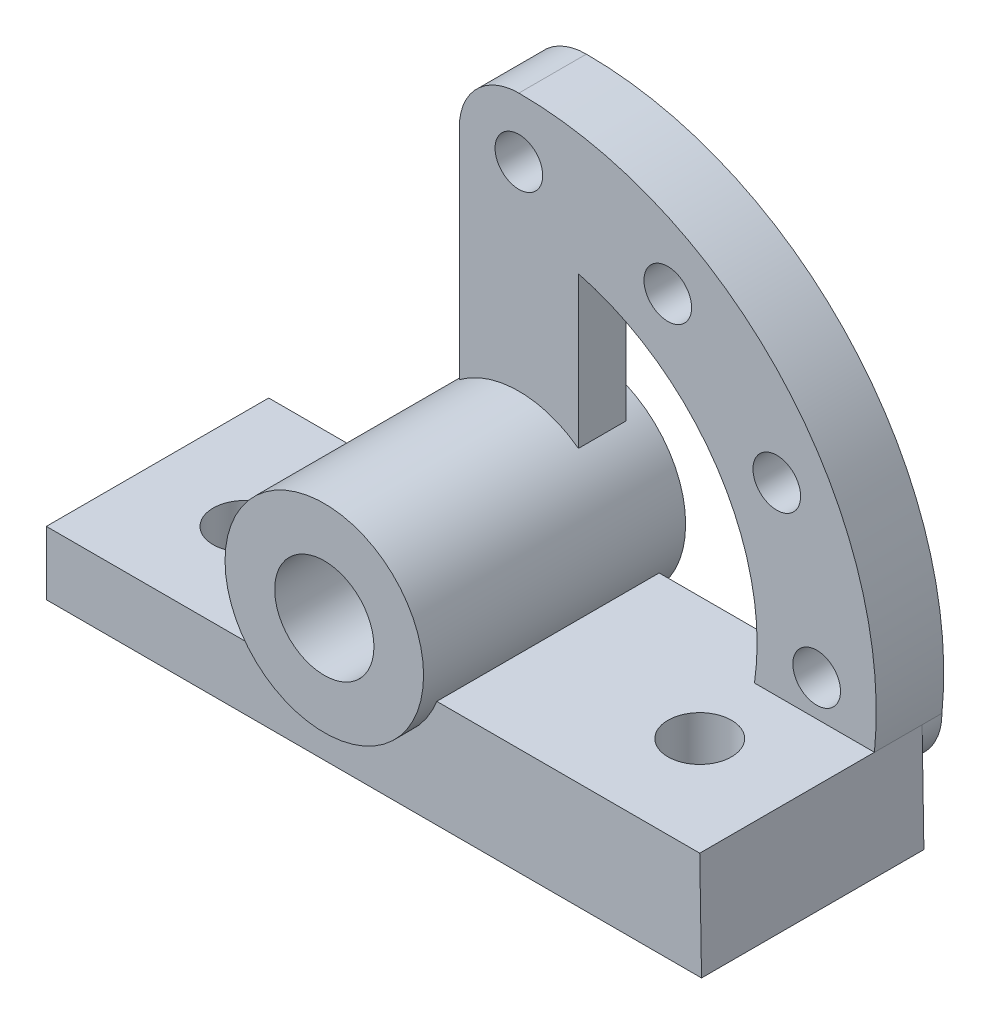
ISO-10303-21;
HEADER;
FILE_DESCRIPTION(('STEP AP214'),'2;1');
FILE_NAME('part.step','',(''),(''),'','','');
FILE_SCHEMA(('AUTOMOTIVE_DESIGN { 1 0 10303 214 1 1 1 1 }'));
ENDSEC;
DATA;
#1=APPLICATION_CONTEXT('core data for automotive mechanical design processes');
#2=APPLICATION_PROTOCOL_DEFINITION('international standard','automotive_design',2000,#1);
#3=PRODUCT_CONTEXT('',#1,'mechanical');
#4=PRODUCT('Part','Part','',(#3));
#5=PRODUCT_RELATED_PRODUCT_CATEGORY('part','',(#4));
#6=PRODUCT_DEFINITION_FORMATION('','',#4);
#7=PRODUCT_DEFINITION_CONTEXT('part definition',#1,'design');
#8=PRODUCT_DEFINITION('design','',#6,#7);
#9=PRODUCT_DEFINITION_SHAPE('','',#8);
#10=(LENGTH_UNIT() NAMED_UNIT(*) SI_UNIT(.MILLI.,.METRE.));
#11=(NAMED_UNIT(*) PLANE_ANGLE_UNIT() SI_UNIT($,.RADIAN.));
#12=(NAMED_UNIT(*) SI_UNIT($,.STERADIAN.) SOLID_ANGLE_UNIT());
#13=UNCERTAINTY_MEASURE_WITH_UNIT(LENGTH_MEASURE(1.E-05),#10,'distance_accuracy_value','');
#14=(GEOMETRIC_REPRESENTATION_CONTEXT(3) GLOBAL_UNCERTAINTY_ASSIGNED_CONTEXT((#13)) GLOBAL_UNIT_ASSIGNED_CONTEXT((#10,
#11,#12)) REPRESENTATION_CONTEXT('',''));
#15=CARTESIAN_POINT('',(0.,0.,0.));
#16=DIRECTION('',(0.,0.,1.));
#17=DIRECTION('',(1.,0.,0.));
#18=AXIS2_PLACEMENT_3D('',#15,#16,#17);
#19=CARTESIAN_POINT('',(75.,36.,-5.));
#20=DIRECTION('',(0.,0.,1.));
#21=DIRECTION('',(1.,0.,0.));
#22=AXIS2_PLACEMENT_3D('',#19,#20,#21);
#23=CYLINDRICAL_SURFACE('',#22,12.5);
#24=CARTESIAN_POINT('',(75.,36.,-5.));
#25=DIRECTION('',(0.,0.,1.));
#26=DIRECTION('',(1.,0.,0.));
#27=AXIS2_PLACEMENT_3D('',#24,#25,#26);
#28=CIRCLE('',#27,12.5);
#29=CARTESIAN_POINT('',(87.5,36.,-5.));
#30=VERTEX_POINT('',#29);
#31=EDGE_CURVE('E313',#30,#30,#28,.T.);
#32=ORIENTED_EDGE('',*,*,#31,.F.);
#33=EDGE_LOOP('',(#32));
#34=FACE_BOUND('',#33,.T.);
#35=CARTESIAN_POINT('',(75.,36.,61.));
#36=DIRECTION('',(0.,0.,1.));
#37=DIRECTION('',(1.,0.,0.));
#38=AXIS2_PLACEMENT_3D('',#35,#36,#37);
#39=CIRCLE('',#38,12.5);
#40=CARTESIAN_POINT('',(87.5,36.,61.));
#41=VERTEX_POINT('',#40);
#42=EDGE_CURVE('E308',#41,#41,#39,.T.);
#43=ORIENTED_EDGE('',*,*,#42,.T.);
#44=EDGE_LOOP('',(#43));
#45=FACE_BOUND('',#44,.T.);
#46=ADVANCED_FACE('F41',(#34,#45),#23,.F.);
#47=CARTESIAN_POINT('',(75.,36.,-5.));
#48=DIRECTION('',(0.,0.,1.));
#49=DIRECTION('',(1.,0.,0.));
#50=AXIS2_PLACEMENT_3D('',#47,#48,#49);
#51=CYLINDRICAL_SURFACE('',#50,25.);
#52=CARTESIAN_POINT('',(75.,36.,12.));
#53=DIRECTION('',(0.,0.,1.));
#54=DIRECTION('',(1.,0.,0.));
#55=AXIS2_PLACEMENT_3D('',#52,#53,#54);
#56=CIRCLE('',#55,25.);
#57=CARTESIAN_POINT('',(90.,56.,12.));
#58=VERTEX_POINT('',#57);
#59=CARTESIAN_POINT('',(60.,56.,12.));
#60=VERTEX_POINT('',#59);
#61=EDGE_CURVE('E171',#58,#60,#56,.T.);
#62=ORIENTED_EDGE('',*,*,#61,.T.);
#63=DIRECTION('',(0.,0.,-1.));
#64=VECTOR('',#63,1.);
#65=CARTESIAN_POINT('',(60.,56.,12.));
#66=LINE('',#65,#64);
#67=CARTESIAN_POINT('',(60.,56.,0.));
#68=VERTEX_POINT('',#67);
#69=EDGE_CURVE('E155',#60,#68,#66,.T.);
#70=ORIENTED_EDGE('',*,*,#69,.T.);
#71=CARTESIAN_POINT('',(75.,36.,0.));
#72=DIRECTION('',(0.,0.,1.));
#73=DIRECTION('',(1.,0.,0.));
#74=AXIS2_PLACEMENT_3D('',#71,#72,#73);
#75=CIRCLE('',#74,25.);
#76=CARTESIAN_POINT('',(90.,56.,0.));
#77=VERTEX_POINT('',#76);
#78=EDGE_CURVE('E192',#77,#68,#75,.T.);
#79=ORIENTED_EDGE('',*,*,#78,.F.);
#80=DIRECTION('',(0.,0.,-1.));
#81=VECTOR('',#80,1.);
#82=CARTESIAN_POINT('',(90.,56.,12.));
#83=LINE('',#82,#81);
#84=EDGE_CURVE('E165',#58,#77,#83,.T.);
#85=ORIENTED_EDGE('',*,*,#84,.F.);
#86=EDGE_LOOP('',(#62,#70,#79,#85));
#87=FACE_BOUND('',#86,.T.);
#88=CARTESIAN_POINT('',(75.,36.,56.));
#89=DIRECTION('',(0.,0.,1.));
#90=DIRECTION('',(1.,0.,0.));
#91=AXIS2_PLACEMENT_3D('',#88,#89,#90);
#92=CIRCLE('',#91,25.);
#93=CARTESIAN_POINT('',(50.,36.,56.));
#94=VERTEX_POINT('',#93);
#95=CARTESIAN_POINT('',(98.3238075793812,27.,56.));
#96=VERTEX_POINT('',#95);
#97=EDGE_CURVE('E258',#94,#96,#92,.T.);
#98=ORIENTED_EDGE('',*,*,#97,.T.);
#99=DIRECTION('',(0.,0.,-1.));
#100=VECTOR('',#99,1.);
#101=CARTESIAN_POINT('',(98.3238075793812,27.,56.));
#102=LINE('',#101,#100);
#103=CARTESIAN_POINT('',(98.3238075793812,27.,0.));
#104=VERTEX_POINT('',#103);
#105=EDGE_CURVE('E305',#96,#104,#102,.T.);
#106=ORIENTED_EDGE('',*,*,#105,.T.);
#107=CARTESIAN_POINT('',(75.,36.,0.));
#108=DIRECTION('',(0.,0.,1.));
#109=DIRECTION('',(1.,0.,0.));
#110=AXIS2_PLACEMENT_3D('',#107,#108,#109);
#111=CIRCLE('',#110,25.);
#112=CARTESIAN_POINT('',(50.,36.,0.));
#113=VERTEX_POINT('',#112);
#114=EDGE_CURVE('E279',#113,#104,#111,.T.);
#115=ORIENTED_EDGE('',*,*,#114,.F.);
#116=DIRECTION('',(0.,0.,-1.));
#117=VECTOR('',#116,1.);
#118=CARTESIAN_POINT('',(50.,36.,56.));
#119=LINE('',#118,#117);
#120=EDGE_CURVE('E299',#94,#113,#119,.T.);
#121=ORIENTED_EDGE('',*,*,#120,.F.);
#122=EDGE_LOOP('',(#98,#106,#115,#121));
#123=FACE_BOUND('',#122,.T.);
#124=CARTESIAN_POINT('',(75.,36.,-5.));
#125=DIRECTION('',(0.,0.,1.));
#126=DIRECTION('',(1.,0.,0.));
#127=AXIS2_PLACEMENT_3D('',#124,#125,#126);
#128=CIRCLE('',#127,25.);
#129=CARTESIAN_POINT('',(100.,36.,-5.));
#130=VERTEX_POINT('',#129);
#131=EDGE_CURVE('E320',#130,#130,#128,.T.);
#132=ORIENTED_EDGE('',*,*,#131,.T.);
#133=EDGE_LOOP('',(#132));
#134=FACE_BOUND('',#133,.T.);
#135=CARTESIAN_POINT('',(75.,36.,61.));
#136=DIRECTION('',(0.,0.,1.));
#137=DIRECTION('',(1.,0.,0.));
#138=AXIS2_PLACEMENT_3D('',#135,#136,#137);
#139=CIRCLE('',#138,25.);
#140=CARTESIAN_POINT('',(100.,36.,61.));
#141=VERTEX_POINT('',#140);
#142=EDGE_CURVE('E311',#141,#141,#139,.T.);
#143=ORIENTED_EDGE('',*,*,#142,.F.);
#144=EDGE_LOOP('',(#143));
#145=FACE_BOUND('',#144,.T.);
#146=ADVANCED_FACE('F177',(#87,#123,#134,#145),#51,.T.);
#147=CARTESIAN_POINT('',(0.,0.,-5.));
#148=DIRECTION('',(0.,0.,1.));
#149=DIRECTION('',(1.,0.,0.));
#150=AXIS2_PLACEMENT_3D('',#147,#148,#149);
#151=PLANE('',#150);
#152=ORIENTED_EDGE('',*,*,#31,.T.);
#153=EDGE_LOOP('',(#152));
#154=FACE_BOUND('',#153,.T.);
#155=ORIENTED_EDGE('',*,*,#131,.F.);
#156=EDGE_LOOP('',(#155));
#157=FACE_BOUND('',#156,.T.);
#158=ADVANCED_FACE('F374',(#154,#157),#151,.F.);
#159=CARTESIAN_POINT('',(0.,0.,61.));
#160=DIRECTION('',(0.,0.,1.));
#161=DIRECTION('',(1.,0.,0.));
#162=AXIS2_PLACEMENT_3D('',#159,#160,#161);
#163=PLANE('',#162);
#164=ORIENTED_EDGE('',*,*,#42,.F.);
#165=EDGE_LOOP('',(#164));
#166=FACE_BOUND('',#165,.T.);
#167=ORIENTED_EDGE('',*,*,#142,.T.);
#168=EDGE_LOOP('',(#167));
#169=FACE_BOUND('',#168,.T.);
#170=ADVANCED_FACE('F379',(#166,#169),#163,.T.);
#171=CARTESIAN_POINT('',(164.953948913937,2.75614014480833,56.));
#172=DIRECTION('',(0.99986044151607,0.0167062111590066,0.));
#173=DIRECTION('',(-0.0167062111590066,0.99986044151607,0.));
#174=AXIS2_PLACEMENT_3D('',#171,#172,#173);
#175=PLANE('',#174);
#176=DIRECTION('',(0.0167062111590066,-0.99986044151607,0.));
#177=VECTOR('',#176,1.);
#178=CARTESIAN_POINT('',(164.953948913937,2.75614014480833,0.));
#179=LINE('',#178,#177);
#180=CARTESIAN_POINT('',(164.548869339596,27.,0.));
#181=VERTEX_POINT('',#180);
#182=CARTESIAN_POINT('',(165.,0.,0.));
#183=VERTEX_POINT('',#182);
#184=EDGE_CURVE('E255',#181,#183,#179,.T.);
#185=ORIENTED_EDGE('',*,*,#184,.F.);
#186=DIRECTION('',(0.,0.,1.));
#187=VECTOR('',#186,1.);
#188=CARTESIAN_POINT('',(164.548869339596,27.,-5.));
#189=LINE('',#188,#187);
#190=CARTESIAN_POINT('',(164.548869339596,27.,12.));
#191=VERTEX_POINT('',#190);
#192=EDGE_CURVE('E248',#181,#191,#189,.T.);
#193=ORIENTED_EDGE('',*,*,#192,.T.);
#194=DIRECTION('',(0.,0.,-1.));
#195=VECTOR('',#194,1.);
#196=CARTESIAN_POINT('',(164.548869339596,27.,56.));
#197=LINE('',#196,#195);
#198=CARTESIAN_POINT('',(164.548869339596,27.,56.));
#199=VERTEX_POINT('',#198);
#200=EDGE_CURVE('E304',#199,#191,#197,.T.);
#201=ORIENTED_EDGE('',*,*,#200,.F.);
#202=DIRECTION('',(0.0167062111590066,-0.99986044151607,0.));
#203=VECTOR('',#202,1.);
#204=CARTESIAN_POINT('',(164.953948913937,2.75614014480833,56.));
#205=LINE('',#204,#203);
#206=CARTESIAN_POINT('',(165.,0.,56.));
#207=VERTEX_POINT('',#206);
#208=EDGE_CURVE('E254',#199,#207,#205,.T.);
#209=ORIENTED_EDGE('',*,*,#208,.T.);
#210=DIRECTION('',(0.,0.,-1.));
#211=VECTOR('',#210,1.);
#212=CARTESIAN_POINT('',(165.,0.,56.));
#213=LINE('',#212,#211);
#214=EDGE_CURVE('E275',#207,#183,#213,.T.);
#215=ORIENTED_EDGE('',*,*,#214,.T.);
#216=EDGE_LOOP('',(#185,#193,#201,#209,#215));
#217=FACE_BOUND('',#216,.T.);
#218=ADVANCED_FACE('F330',(#217),#175,.T.);
#219=CARTESIAN_POINT('',(0.,27.,56.));
#220=DIRECTION('',(0.,1.,0.));
#221=DIRECTION('',(0.,0.,1.));
#222=AXIS2_PLACEMENT_3D('',#219,#220,#221);
#223=PLANE('',#222);
#224=CARTESIAN_POINT('',(139.548869339596,27.,31.));
#225=DIRECTION('',(0.,1.,0.));
#226=DIRECTION('',(0.,0.,1.));
#227=AXIS2_PLACEMENT_3D('',#224,#225,#226);
#228=CIRCLE('',#227,8.00000000000001);
#229=CARTESIAN_POINT('',(139.548869339596,27.,39.));
#230=VERTEX_POINT('',#229);
#231=EDGE_CURVE('E186',#230,#230,#228,.F.);
#232=ORIENTED_EDGE('',*,*,#231,.T.);
#233=EDGE_LOOP('',(#232));
#234=FACE_BOUND('',#233,.T.);
#235=DIRECTION('',(0.,0.,1.));
#236=VECTOR('',#235,1.);
#237=CARTESIAN_POINT('',(134.367214412294,27.,-5.));
#238=LINE('',#237,#236);
#239=CARTESIAN_POINT('',(134.367214412294,27.,0.));
#240=VERTEX_POINT('',#239);
#241=CARTESIAN_POINT('',(134.367214412294,27.,12.));
#242=VERTEX_POINT('',#241);
#243=EDGE_CURVE('E242',#240,#242,#238,.T.);
#244=ORIENTED_EDGE('',*,*,#243,.F.);
#245=DIRECTION('',(1.,0.,0.));
#246=VECTOR('',#245,1.);
#247=CARTESIAN_POINT('',(0.,27.,0.));
#248=LINE('',#247,#246);
#249=EDGE_CURVE('E273',#104,#240,#248,.T.);
#250=ORIENTED_EDGE('',*,*,#249,.F.);
#251=ORIENTED_EDGE('',*,*,#105,.F.);
#252=DIRECTION('',(1.,0.,0.));
#253=VECTOR('',#252,1.);
#254=CARTESIAN_POINT('',(0.,27.,56.));
#255=LINE('',#254,#253);
#256=EDGE_CURVE('E257',#96,#199,#255,.T.);
#257=ORIENTED_EDGE('',*,*,#256,.T.);
#258=ORIENTED_EDGE('',*,*,#200,.T.);
#259=DIRECTION('',(1.,0.,0.));
#260=VECTOR('',#259,1.);
#261=CARTESIAN_POINT('',(0.,27.,12.));
#262=LINE('',#261,#260);
#263=EDGE_CURVE('E11',#242,#191,#262,.T.);
#264=ORIENTED_EDGE('',*,*,#263,.F.);
#265=EDGE_LOOP('',(#244,#250,#251,#257,#258,#264));
#266=FACE_BOUND('',#265,.T.);
#267=ADVANCED_FACE('F353',(#234,#266),#223,.T.);
#268=CARTESIAN_POINT('',(50.,0.,56.));
#269=DIRECTION('',(1.,0.,0.));
#270=DIRECTION('',(0.,0.,-1.));
#271=AXIS2_PLACEMENT_3D('',#268,#269,#270);
#272=PLANE('',#271);
#273=DIRECTION('',(0.,-1.,0.));
#274=VECTOR('',#273,1.);
#275=CARTESIAN_POINT('',(50.,0.,0.));
#276=LINE('',#275,#274);
#277=CARTESIAN_POINT('',(50.,16.,0.));
#278=VERTEX_POINT('',#277);
#279=EDGE_CURVE('E284',#113,#278,#276,.T.);
#280=ORIENTED_EDGE('',*,*,#279,.T.);
#281=DIRECTION('',(0.,0.,-1.));
#282=VECTOR('',#281,1.);
#283=CARTESIAN_POINT('',(50.,16.,56.));
#284=LINE('',#283,#282);
#285=CARTESIAN_POINT('',(50.,16.,56.));
#286=VERTEX_POINT('',#285);
#287=EDGE_CURVE('E298',#286,#278,#284,.T.);
#288=ORIENTED_EDGE('',*,*,#287,.F.);
#289=DIRECTION('',(0.,-1.,0.));
#290=VECTOR('',#289,1.);
#291=CARTESIAN_POINT('',(50.,0.,56.));
#292=LINE('',#291,#290);
#293=EDGE_CURVE('E265',#94,#286,#292,.T.);
#294=ORIENTED_EDGE('',*,*,#293,.F.);
#295=ORIENTED_EDGE('',*,*,#120,.T.);
#296=EDGE_LOOP('',(#280,#288,#294,#295));
#297=FACE_BOUND('',#296,.T.);
#298=ADVANCED_FACE('F350',(#297),#272,.F.);
#299=CARTESIAN_POINT('',(0.,16.,56.));
#300=DIRECTION('',(0.,-1.,0.));
#301=DIRECTION('',(0.,0.,-1.));
#302=AXIS2_PLACEMENT_3D('',#299,#300,#301);
#303=PLANE('',#302);
#304=CARTESIAN_POINT('',(25.,16.,31.));
#305=DIRECTION('',(0.,-1.,0.));
#306=DIRECTION('',(0.,0.,-1.));
#307=AXIS2_PLACEMENT_3D('',#304,#305,#306);
#308=CIRCLE('',#307,8.);
#309=CARTESIAN_POINT('',(25.,16.,23.));
#310=VERTEX_POINT('',#309);
#311=EDGE_CURVE('E666',#310,#310,#308,.F.);
#312=ORIENTED_EDGE('',*,*,#311,.F.);
#313=EDGE_LOOP('',(#312));
#314=FACE_BOUND('',#313,.T.);
#315=DIRECTION('',(-1.,0.,0.));
#316=VECTOR('',#315,1.);
#317=CARTESIAN_POINT('',(0.,16.,0.));
#318=LINE('',#317,#316);
#319=CARTESIAN_POINT('',(0.,16.,0.));
#320=VERTEX_POINT('',#319);
#321=EDGE_CURVE('E285',#278,#320,#318,.T.);
#322=ORIENTED_EDGE('',*,*,#321,.T.);
#323=DIRECTION('',(0.,0.,-1.));
#324=VECTOR('',#323,1.);
#325=CARTESIAN_POINT('',(0.,16.,56.));
#326=LINE('',#325,#324);
#327=CARTESIAN_POINT('',(0.,16.,56.));
#328=VERTEX_POINT('',#327);
#329=EDGE_CURVE('E295',#328,#320,#326,.T.);
#330=ORIENTED_EDGE('',*,*,#329,.F.);
#331=DIRECTION('',(-1.,0.,0.));
#332=VECTOR('',#331,1.);
#333=CARTESIAN_POINT('',(0.,16.,56.));
#334=LINE('',#333,#332);
#335=EDGE_CURVE('E262',#286,#328,#334,.T.);
#336=ORIENTED_EDGE('',*,*,#335,.F.);
#337=ORIENTED_EDGE('',*,*,#287,.T.);
#338=EDGE_LOOP('',(#322,#330,#336,#337));
#339=FACE_BOUND('',#338,.T.);
#340=ADVANCED_FACE('F344',(#314,#339),#303,.F.);
#341=CARTESIAN_POINT('',(0.,0.,56.));
#342=DIRECTION('',(-1.,0.,0.));
#343=DIRECTION('',(0.,0.,1.));
#344=AXIS2_PLACEMENT_3D('',#341,#342,#343);
#345=PLANE('',#344);
#346=DIRECTION('',(0.,1.,0.));
#347=VECTOR('',#346,1.);
#348=CARTESIAN_POINT('',(0.,0.,0.));
#349=LINE('',#348,#347);
#350=CARTESIAN_POINT('',(0.,0.,0.));
#351=VERTEX_POINT('',#350);
#352=EDGE_CURVE('E286',#351,#320,#349,.T.);
#353=ORIENTED_EDGE('',*,*,#352,.F.);
#354=DIRECTION('',(0.,0.,-1.));
#355=VECTOR('',#354,1.);
#356=CARTESIAN_POINT('',(0.,0.,56.));
#357=LINE('',#356,#355);
#358=CARTESIAN_POINT('',(0.,0.,56.));
#359=VERTEX_POINT('',#358);
#360=EDGE_CURVE('E292',#359,#351,#357,.T.);
#361=ORIENTED_EDGE('',*,*,#360,.F.);
#362=DIRECTION('',(0.,1.,0.));
#363=VECTOR('',#362,1.);
#364=CARTESIAN_POINT('',(0.,0.,56.));
#365=LINE('',#364,#363);
#366=EDGE_CURVE('E270',#359,#328,#365,.T.);
#367=ORIENTED_EDGE('',*,*,#366,.T.);
#368=ORIENTED_EDGE('',*,*,#329,.T.);
#369=EDGE_LOOP('',(#353,#361,#367,#368));
#370=FACE_BOUND('',#369,.T.);
#371=ADVANCED_FACE('F336',(#370),#345,.T.);
#372=CARTESIAN_POINT('',(0.,0.,56.));
#373=DIRECTION('',(0.,1.,0.));
#374=DIRECTION('',(0.,0.,1.));
#375=AXIS2_PLACEMENT_3D('',#372,#373,#374);
#376=PLANE('',#375);
#377=CARTESIAN_POINT('',(139.548869339596,0.,31.));
#378=DIRECTION('',(0.,1.,0.));
#379=DIRECTION('',(0.,0.,1.));
#380=AXIS2_PLACEMENT_3D('',#377,#378,#379);
#381=CIRCLE('',#380,8.00000000000001);
#382=CARTESIAN_POINT('',(139.548869339596,0.,39.));
#383=VERTEX_POINT('',#382);
#384=EDGE_CURVE('E669',#383,#383,#381,.T.);
#385=ORIENTED_EDGE('',*,*,#384,.T.);
#386=EDGE_LOOP('',(#385));
#387=FACE_BOUND('',#386,.T.);
#388=CARTESIAN_POINT('',(25.,0.,31.));
#389=DIRECTION('',(0.,1.,0.));
#390=DIRECTION('',(0.,0.,1.));
#391=AXIS2_PLACEMENT_3D('',#388,#389,#390);
#392=CIRCLE('',#391,8.);
#393=CARTESIAN_POINT('',(25.,0.,39.));
#394=VERTEX_POINT('',#393);
#395=EDGE_CURVE('E668',#394,#394,#392,.T.);
#396=ORIENTED_EDGE('',*,*,#395,.T.);
#397=EDGE_LOOP('',(#396));
#398=FACE_BOUND('',#397,.T.);
#399=DIRECTION('',(1.,0.,0.));
#400=VECTOR('',#399,1.);
#401=CARTESIAN_POINT('',(0.,0.,0.));
#402=LINE('',#401,#400);
#403=EDGE_CURVE('E260',#351,#183,#402,.T.);
#404=ORIENTED_EDGE('',*,*,#403,.T.);
#405=ORIENTED_EDGE('',*,*,#214,.F.);
#406=DIRECTION('',(1.,0.,0.));
#407=VECTOR('',#406,1.);
#408=CARTESIAN_POINT('',(0.,0.,56.));
#409=LINE('',#408,#407);
#410=EDGE_CURVE('E269',#359,#207,#409,.T.);
#411=ORIENTED_EDGE('',*,*,#410,.F.);
#412=ORIENTED_EDGE('',*,*,#360,.T.);
#413=EDGE_LOOP('',(#404,#405,#411,#412));
#414=FACE_BOUND('',#413,.T.);
#415=ADVANCED_FACE('F332',(#387,#398,#414),#376,.F.);
#416=CARTESIAN_POINT('',(0.,0.,56.));
#417=DIRECTION('',(0.,0.,1.));
#418=DIRECTION('',(1.,0.,0.));
#419=AXIS2_PLACEMENT_3D('',#416,#417,#418);
#420=PLANE('',#419);
#421=ORIENTED_EDGE('',*,*,#208,.F.);
#422=ORIENTED_EDGE('',*,*,#256,.F.);
#423=ORIENTED_EDGE('',*,*,#97,.F.);
#424=ORIENTED_EDGE('',*,*,#293,.T.);
#425=ORIENTED_EDGE('',*,*,#335,.T.);
#426=ORIENTED_EDGE('',*,*,#366,.F.);
#427=ORIENTED_EDGE('',*,*,#410,.T.);
#428=EDGE_LOOP('',(#421,#422,#423,#424,#425,#426,#427));
#429=FACE_BOUND('',#428,.T.);
#430=ADVANCED_FACE('F354',(#429),#420,.T.);
#431=CARTESIAN_POINT('',(0.,0.,0.));
#432=DIRECTION('',(0.,0.,1.));
#433=DIRECTION('',(1.,0.,0.));
#434=AXIS2_PLACEMENT_3D('',#431,#432,#433);
#435=PLANE('',#434);
#436=ORIENTED_EDGE('',*,*,#249,.T.);
#437=CARTESIAN_POINT('',(149.458041875945,27.,0.));
#438=DIRECTION('',(0.,0.,1.));
#439=DIRECTION('',(1.,0.,0.));
#440=AXIS2_PLACEMENT_3D('',#437,#438,#439);
#441=CIRCLE('',#440,15.0908274636506);
#442=EDGE_CURVE('E48',#240,#181,#441,.T.);
#443=ORIENTED_EDGE('',*,*,#442,.T.);
#444=ORIENTED_EDGE('',*,*,#184,.T.);
#445=ORIENTED_EDGE('',*,*,#403,.F.);
#446=ORIENTED_EDGE('',*,*,#352,.T.);
#447=ORIENTED_EDGE('',*,*,#321,.F.);
#448=ORIENTED_EDGE('',*,*,#279,.F.);
#449=ORIENTED_EDGE('',*,*,#114,.T.);
#450=EDGE_LOOP('',(#436,#443,#444,#445,#446,#447,#448,#449));
#451=FACE_BOUND('',#450,.T.);
#452=ADVANCED_FACE('F325',(#451),#435,.F.);
#453=CARTESIAN_POINT('',(75.,36.,-5.));
#454=DIRECTION('',(0.,0.,1.));
#455=DIRECTION('',(1.,0.,0.));
#456=AXIS2_PLACEMENT_3D('',#453,#454,#455);
#457=CYLINDRICAL_SURFACE('',#456,60.);
#458=CARTESIAN_POINT('',(75.,36.,12.));
#459=DIRECTION('',(0.,0.,1.));
#460=DIRECTION('',(1.,0.,0.));
#461=AXIS2_PLACEMENT_3D('',#458,#459,#460);
#462=CIRCLE('',#461,60.);
#463=CARTESIAN_POINT('',(134.370917994373,27.3343150007925,12.));
#464=VERTEX_POINT('',#463);
#465=CARTESIAN_POINT('',(90.,94.0947501931113,12.));
#466=VERTEX_POINT('',#465);
#467=EDGE_CURVE('E208',#464,#466,#462,.T.);
#468=ORIENTED_EDGE('',*,*,#467,.T.);
#469=DIRECTION('',(0.,0.,-1.));
#470=VECTOR('',#469,1.);
#471=CARTESIAN_POINT('',(90.,94.0947501931113,12.));
#472=LINE('',#471,#470);
#473=CARTESIAN_POINT('',(90.,94.0947501931113,0.));
#474=VERTEX_POINT('',#473);
#475=EDGE_CURVE('E64',#466,#474,#472,.T.);
#476=ORIENTED_EDGE('',*,*,#475,.T.);
#477=CARTESIAN_POINT('',(75.,36.,0.));
#478=DIRECTION('',(0.,0.,1.));
#479=DIRECTION('',(1.,0.,0.));
#480=AXIS2_PLACEMENT_3D('',#477,#478,#479);
#481=CIRCLE('',#480,60.);
#482=CARTESIAN_POINT('',(75.,96.,0.));
#483=VERTEX_POINT('',#482);
#484=EDGE_CURVE('E176',#474,#483,#481,.T.);
#485=ORIENTED_EDGE('',*,*,#484,.T.);
#486=DIRECTION('',(0.,0.,1.));
#487=VECTOR('',#486,1.);
#488=CARTESIAN_POINT('',(75.,96.,-5.));
#489=LINE('',#488,#487);
#490=CARTESIAN_POINT('',(75.,96.,-5.));
#491=VERTEX_POINT('',#490);
#492=EDGE_CURVE('E241',#491,#483,#489,.T.);
#493=ORIENTED_EDGE('',*,*,#492,.F.);
#494=CARTESIAN_POINT('',(75.,36.,-5.));
#495=DIRECTION('',(0.,0.,1.));
#496=DIRECTION('',(1.,0.,0.));
#497=AXIS2_PLACEMENT_3D('',#494,#495,#496);
#498=CIRCLE('',#497,60.);
#499=CARTESIAN_POINT('',(134.370917994373,27.3343150007925,-5.));
#500=VERTEX_POINT('',#499);
#501=EDGE_CURVE('E230',#500,#491,#498,.T.);
#502=ORIENTED_EDGE('',*,*,#501,.F.);
#503=DIRECTION('',(0.,0.,1.));
#504=VECTOR('',#503,1.);
#505=CARTESIAN_POINT('',(134.370917994373,27.3343150007925,-5.));
#506=LINE('',#505,#504);
#507=EDGE_CURVE('E239',#500,#464,#506,.T.);
#508=ORIENTED_EDGE('',*,*,#507,.T.);
#509=EDGE_LOOP('',(#468,#476,#485,#493,#502,#508));
#510=FACE_BOUND('',#509,.T.);
#511=ADVANCED_FACE('F361',(#510),#457,.F.);
#512=CARTESIAN_POINT('',(75.,111.,-5.));
#513=DIRECTION('',(0.,0.,1.));
#514=DIRECTION('',(1.,0.,0.));
#515=AXIS2_PLACEMENT_3D('',#512,#513,#514);
#516=CYLINDRICAL_SURFACE('',#515,15.);
#517=DIRECTION('',(0.,0.,-1.));
#518=VECTOR('',#517,1.);
#519=CARTESIAN_POINT('',(60.,111.,12.));
#520=LINE('',#519,#518);
#521=CARTESIAN_POINT('',(60.,111.,12.));
#522=VERTEX_POINT('',#521);
#523=CARTESIAN_POINT('',(60.,111.,0.));
#524=VERTEX_POINT('',#523);
#525=EDGE_CURVE('E161',#522,#524,#520,.T.);
#526=ORIENTED_EDGE('',*,*,#525,.F.);
#527=CARTESIAN_POINT('',(75.,111.,12.));
#528=DIRECTION('',(0.,0.,1.));
#529=DIRECTION('',(1.,0.,0.));
#530=AXIS2_PLACEMENT_3D('',#527,#528,#529);
#531=CIRCLE('',#530,15.);
#532=CARTESIAN_POINT('',(75.,126.,12.));
#533=VERTEX_POINT('',#532);
#534=EDGE_CURVE('E174',#533,#522,#531,.T.);
#535=ORIENTED_EDGE('',*,*,#534,.F.);
#536=DIRECTION('',(0.,0.,1.));
#537=VECTOR('',#536,1.);
#538=CARTESIAN_POINT('',(75.,126.,-5.));
#539=LINE('',#538,#537);
#540=CARTESIAN_POINT('',(75.,126.,-5.));
#541=VERTEX_POINT('',#540);
#542=EDGE_CURVE('E244',#541,#533,#539,.T.);
#543=ORIENTED_EDGE('',*,*,#542,.F.);
#544=CARTESIAN_POINT('',(75.,111.,-5.));
#545=DIRECTION('',(0.,0.,1.));
#546=DIRECTION('',(1.,0.,0.));
#547=AXIS2_PLACEMENT_3D('',#544,#545,#546);
#548=CIRCLE('',#547,15.);
#549=EDGE_CURVE('E240',#541,#491,#548,.T.);
#550=ORIENTED_EDGE('',*,*,#549,.T.);
#551=ORIENTED_EDGE('',*,*,#492,.T.);
#552=CARTESIAN_POINT('',(75.,111.,0.));
#553=DIRECTION('',(0.,0.,1.));
#554=DIRECTION('',(1.,0.,0.));
#555=AXIS2_PLACEMENT_3D('',#552,#553,#554);
#556=CIRCLE('',#555,15.);
#557=EDGE_CURVE('E187',#524,#483,#556,.T.);
#558=ORIENTED_EDGE('',*,*,#557,.F.);
#559=EDGE_LOOP('',(#526,#535,#543,#550,#551,#558));
#560=FACE_BOUND('',#559,.T.);
#561=ADVANCED_FACE('F542',(#560),#516,.T.);
#562=CARTESIAN_POINT('',(75.,36.,-5.));
#563=DIRECTION('',(0.,0.,1.));
#564=DIRECTION('',(1.,0.,0.));
#565=AXIS2_PLACEMENT_3D('',#562,#563,#564);
#566=CYLINDRICAL_SURFACE('',#565,90.);
#567=ORIENTED_EDGE('',*,*,#542,.T.);
#568=CARTESIAN_POINT('',(75.,36.,12.));
#569=DIRECTION('',(0.,0.,1.));
#570=DIRECTION('',(1.,0.,0.));
#571=AXIS2_PLACEMENT_3D('',#568,#569,#570);
#572=CIRCLE('',#571,90.);
#573=EDGE_CURVE('E211',#191,#533,#572,.T.);
#574=ORIENTED_EDGE('',*,*,#573,.F.);
#575=ORIENTED_EDGE('',*,*,#192,.F.);
#576=CARTESIAN_POINT('',(164.548869339596,27.,-5.));
#577=VERTEX_POINT('',#576);
#578=EDGE_CURVE('E250',#577,#181,#189,.T.);
#579=ORIENTED_EDGE('',*,*,#578,.F.);
#580=CARTESIAN_POINT('',(75.,36.,-5.));
#581=DIRECTION('',(0.,0.,1.));
#582=DIRECTION('',(1.,0.,0.));
#583=AXIS2_PLACEMENT_3D('',#580,#581,#582);
#584=CIRCLE('',#583,90.);
#585=EDGE_CURVE('E234',#577,#541,#584,.T.);
#586=ORIENTED_EDGE('',*,*,#585,.T.);
#587=EDGE_LOOP('',(#567,#574,#575,#579,#586));
#588=FACE_BOUND('',#587,.T.);
#589=ADVANCED_FACE('F537',(#588),#566,.T.);
#590=CARTESIAN_POINT('',(75.,111.,-5.));
#591=DIRECTION('',(0.,0.,1.));
#592=DIRECTION('',(1.,0.,0.));
#593=AXIS2_PLACEMENT_3D('',#590,#591,#592);
#594=CYLINDRICAL_SURFACE('',#593,6.);
#595=CARTESIAN_POINT('',(75.,111.,-5.));
#596=DIRECTION('',(0.,0.,1.));
#597=DIRECTION('',(1.,0.,0.));
#598=AXIS2_PLACEMENT_3D('',#595,#596,#597);
#599=CIRCLE('',#598,6.);
#600=CARTESIAN_POINT('',(81.,111.,-5.));
#601=VERTEX_POINT('',#600);
#602=EDGE_CURVE('E228',#601,#601,#599,.T.);
#603=ORIENTED_EDGE('',*,*,#602,.F.);
#604=EDGE_LOOP('',(#603));
#605=FACE_BOUND('',#604,.T.);
#606=CARTESIAN_POINT('',(75.,111.,12.));
#607=DIRECTION('',(0.,0.,1.));
#608=DIRECTION('',(1.,0.,0.));
#609=AXIS2_PLACEMENT_3D('',#606,#607,#608);
#610=CIRCLE('',#609,6.);
#611=CARTESIAN_POINT('',(81.,111.,12.));
#612=VERTEX_POINT('',#611);
#613=EDGE_CURVE('E210',#612,#612,#610,.T.);
#614=ORIENTED_EDGE('',*,*,#613,.T.);
#615=EDGE_LOOP('',(#614));
#616=FACE_BOUND('',#615,.T.);
#617=ADVANCED_FACE('F530',(#605,#616),#594,.F.);
#618=CARTESIAN_POINT('',(150.,36.,-5.));
#619=DIRECTION('',(0.,0.,1.));
#620=DIRECTION('',(1.,0.,0.));
#621=AXIS2_PLACEMENT_3D('',#618,#619,#620);
#622=CYLINDRICAL_SURFACE('',#621,5.99999999999999);
#623=CARTESIAN_POINT('',(150.,36.,-5.));
#624=DIRECTION('',(0.,0.,1.));
#625=DIRECTION('',(1.,0.,0.));
#626=AXIS2_PLACEMENT_3D('',#623,#624,#625);
#627=CIRCLE('',#626,5.99999999999999);
#628=CARTESIAN_POINT('',(156.,36.,-5.));
#629=VERTEX_POINT('',#628);
#630=EDGE_CURVE('E223',#629,#629,#627,.T.);
#631=ORIENTED_EDGE('',*,*,#630,.F.);
#632=EDGE_LOOP('',(#631));
#633=FACE_BOUND('',#632,.T.);
#634=CARTESIAN_POINT('',(150.,36.,12.));
#635=DIRECTION('',(0.,0.,1.));
#636=DIRECTION('',(1.,0.,0.));
#637=AXIS2_PLACEMENT_3D('',#634,#635,#636);
#638=CIRCLE('',#637,5.99999999999999);
#639=CARTESIAN_POINT('',(156.,36.,12.));
#640=VERTEX_POINT('',#639);
#641=EDGE_CURVE('E202',#640,#640,#638,.T.);
#642=ORIENTED_EDGE('',*,*,#641,.T.);
#643=EDGE_LOOP('',(#642));
#644=FACE_BOUND('',#643,.T.);
#645=ADVANCED_FACE('F519',(#633,#644),#622,.F.);
#646=CARTESIAN_POINT('',(112.5,100.951905283833,-5.));
#647=DIRECTION('',(0.,0.,1.));
#648=DIRECTION('',(1.,0.,0.));
#649=AXIS2_PLACEMENT_3D('',#646,#647,#648);
#650=CYLINDRICAL_SURFACE('',#649,6.);
#651=CARTESIAN_POINT('',(112.5,100.951905283833,-5.));
#652=DIRECTION('',(0.,0.,1.));
#653=DIRECTION('',(1.,0.,0.));
#654=AXIS2_PLACEMENT_3D('',#651,#652,#653);
#655=CIRCLE('',#654,6.);
#656=CARTESIAN_POINT('',(118.5,100.951905283833,-5.));
#657=VERTEX_POINT('',#656);
#658=EDGE_CURVE('E217',#657,#657,#655,.T.);
#659=ORIENTED_EDGE('',*,*,#658,.F.);
#660=EDGE_LOOP('',(#659));
#661=FACE_BOUND('',#660,.T.);
#662=CARTESIAN_POINT('',(112.5,100.951905283833,12.));
#663=DIRECTION('',(0.,0.,1.));
#664=DIRECTION('',(1.,0.,0.));
#665=AXIS2_PLACEMENT_3D('',#662,#663,#664);
#666=CIRCLE('',#665,6.);
#667=CARTESIAN_POINT('',(118.5,100.951905283833,12.));
#668=VERTEX_POINT('',#667);
#669=EDGE_CURVE('E201',#668,#668,#666,.T.);
#670=ORIENTED_EDGE('',*,*,#669,.T.);
#671=EDGE_LOOP('',(#670));
#672=FACE_BOUND('',#671,.T.);
#673=ADVANCED_FACE('F509',(#661,#672),#650,.F.);
#674=CARTESIAN_POINT('',(139.951905283833,73.5000000000001,-5.));
#675=DIRECTION('',(0.,0.,1.));
#676=DIRECTION('',(1.,0.,0.));
#677=AXIS2_PLACEMENT_3D('',#674,#675,#676);
#678=CYLINDRICAL_SURFACE('',#677,5.99999999999999);
#679=CARTESIAN_POINT('',(139.951905283833,73.5000000000001,-5.));
#680=DIRECTION('',(0.,0.,1.));
#681=DIRECTION('',(1.,0.,0.));
#682=AXIS2_PLACEMENT_3D('',#679,#680,#681);
#683=CIRCLE('',#682,5.99999999999999);
#684=CARTESIAN_POINT('',(145.951905283833,73.5000000000001,-5.));
#685=VERTEX_POINT('',#684);
#686=EDGE_CURVE('E216',#685,#685,#683,.T.);
#687=ORIENTED_EDGE('',*,*,#686,.F.);
#688=EDGE_LOOP('',(#687));
#689=FACE_BOUND('',#688,.T.);
#690=CARTESIAN_POINT('',(139.951905283833,73.5000000000001,12.));
#691=DIRECTION('',(0.,0.,1.));
#692=DIRECTION('',(1.,0.,0.));
#693=AXIS2_PLACEMENT_3D('',#690,#691,#692);
#694=CIRCLE('',#693,5.99999999999999);
#695=CARTESIAN_POINT('',(145.951905283833,73.5000000000001,12.));
#696=VERTEX_POINT('',#695);
#697=EDGE_CURVE('E200',#696,#696,#694,.T.);
#698=ORIENTED_EDGE('',*,*,#697,.T.);
#699=EDGE_LOOP('',(#698));
#700=FACE_BOUND('',#699,.T.);
#701=ADVANCED_FACE('F505',(#689,#700),#678,.F.);
#702=CARTESIAN_POINT('',(149.458041875945,27.,-5.));
#703=DIRECTION('',(0.,0.,1.));
#704=DIRECTION('',(1.,0.,0.));
#705=AXIS2_PLACEMENT_3D('',#702,#703,#704);
#706=CYLINDRICAL_SURFACE('',#705,15.0908274636506);
#707=ORIENTED_EDGE('',*,*,#442,.F.);
#708=ORIENTED_EDGE('',*,*,#243,.T.);
#709=CARTESIAN_POINT('',(149.458041875945,27.,12.));
#710=DIRECTION('',(0.,0.,1.));
#711=DIRECTION('',(1.,0.,0.));
#712=AXIS2_PLACEMENT_3D('',#709,#710,#711);
#713=CIRCLE('',#712,15.0908274636506);
#714=EDGE_CURVE('E215',#464,#242,#713,.T.);
#715=ORIENTED_EDGE('',*,*,#714,.F.);
#716=ORIENTED_EDGE('',*,*,#507,.F.);
#717=CARTESIAN_POINT('',(149.458041875945,27.,-5.));
#718=DIRECTION('',(0.,0.,1.));
#719=DIRECTION('',(1.,0.,0.));
#720=AXIS2_PLACEMENT_3D('',#717,#718,#719);
#721=CIRCLE('',#720,15.0908274636506);
#722=EDGE_CURVE('E233',#500,#577,#721,.T.);
#723=ORIENTED_EDGE('',*,*,#722,.T.);
#724=ORIENTED_EDGE('',*,*,#578,.T.);
#725=EDGE_LOOP('',(#707,#708,#715,#716,#723,#724));
#726=FACE_BOUND('',#725,.T.);
#727=ADVANCED_FACE('F491',(#726),#706,.T.);
#728=CARTESIAN_POINT('',(0.,0.,-5.));
#729=DIRECTION('',(0.,0.,1.));
#730=DIRECTION('',(1.,0.,0.));
#731=AXIS2_PLACEMENT_3D('',#728,#729,#730);
#732=PLANE('',#731);
#733=ORIENTED_EDGE('',*,*,#686,.T.);
#734=EDGE_LOOP('',(#733));
#735=FACE_BOUND('',#734,.T.);
#736=ORIENTED_EDGE('',*,*,#658,.T.);
#737=EDGE_LOOP('',(#736));
#738=FACE_BOUND('',#737,.T.);
#739=ORIENTED_EDGE('',*,*,#630,.T.);
#740=EDGE_LOOP('',(#739));
#741=FACE_BOUND('',#740,.T.);
#742=ORIENTED_EDGE('',*,*,#602,.T.);
#743=EDGE_LOOP('',(#742));
#744=FACE_BOUND('',#743,.T.);
#745=ORIENTED_EDGE('',*,*,#501,.T.);
#746=ORIENTED_EDGE('',*,*,#549,.F.);
#747=ORIENTED_EDGE('',*,*,#585,.F.);
#748=ORIENTED_EDGE('',*,*,#722,.F.);
#749=EDGE_LOOP('',(#745,#746,#747,#748));
#750=FACE_BOUND('',#749,.T.);
#751=ADVANCED_FACE('F485',(#735,#738,#741,#744,#750),#732,.F.);
#752=CARTESIAN_POINT('',(0.,0.,12.));
#753=DIRECTION('',(0.,0.,1.));
#754=DIRECTION('',(1.,0.,0.));
#755=AXIS2_PLACEMENT_3D('',#752,#753,#754);
#756=PLANE('',#755);
#757=ORIENTED_EDGE('',*,*,#697,.F.);
#758=EDGE_LOOP('',(#757));
#759=FACE_BOUND('',#758,.T.);
#760=ORIENTED_EDGE('',*,*,#669,.F.);
#761=EDGE_LOOP('',(#760));
#762=FACE_BOUND('',#761,.T.);
#763=ORIENTED_EDGE('',*,*,#641,.F.);
#764=EDGE_LOOP('',(#763));
#765=FACE_BOUND('',#764,.T.);
#766=ORIENTED_EDGE('',*,*,#613,.F.);
#767=EDGE_LOOP('',(#766));
#768=FACE_BOUND('',#767,.T.);
#769=ORIENTED_EDGE('',*,*,#714,.T.);
#770=ORIENTED_EDGE('',*,*,#263,.T.);
#771=ORIENTED_EDGE('',*,*,#573,.T.);
#772=ORIENTED_EDGE('',*,*,#534,.T.);
#773=DIRECTION('',(0.,1.,0.));
#774=VECTOR('',#773,1.);
#775=CARTESIAN_POINT('',(60.,0.,12.));
#776=LINE('',#775,#774);
#777=EDGE_CURVE('E160',#60,#522,#776,.T.);
#778=ORIENTED_EDGE('',*,*,#777,.F.);
#779=ORIENTED_EDGE('',*,*,#61,.F.);
#780=DIRECTION('',(0.,-1.,0.));
#781=VECTOR('',#780,1.);
#782=CARTESIAN_POINT('',(90.,0.,12.));
#783=LINE('',#782,#781);
#784=EDGE_CURVE('E181',#466,#58,#783,.T.);
#785=ORIENTED_EDGE('',*,*,#784,.F.);
#786=ORIENTED_EDGE('',*,*,#467,.F.);
#787=EDGE_LOOP('',(#769,#770,#771,#772,#778,#779,#785,#786));
#788=FACE_BOUND('',#787,.T.);
#789=ADVANCED_FACE('F169',(#759,#762,#765,#768,#788),#756,.T.);
#790=CARTESIAN_POINT('',(60.,0.,12.));
#791=DIRECTION('',(-1.,0.,0.));
#792=DIRECTION('',(0.,0.,1.));
#793=AXIS2_PLACEMENT_3D('',#790,#791,#792);
#794=PLANE('',#793);
#795=DIRECTION('',(0.,1.,0.));
#796=VECTOR('',#795,1.);
#797=CARTESIAN_POINT('',(60.,0.,0.));
#798=LINE('',#797,#796);
#799=EDGE_CURVE('E157',#68,#524,#798,.T.);
#800=ORIENTED_EDGE('',*,*,#799,.F.);
#801=ORIENTED_EDGE('',*,*,#69,.F.);
#802=ORIENTED_EDGE('',*,*,#777,.T.);
#803=ORIENTED_EDGE('',*,*,#525,.T.);
#804=EDGE_LOOP('',(#800,#801,#802,#803));
#805=FACE_BOUND('',#804,.T.);
#806=ADVANCED_FACE('F152',(#805),#794,.T.);
#807=CARTESIAN_POINT('',(90.,0.,12.));
#808=DIRECTION('',(1.,0.,0.));
#809=DIRECTION('',(0.,0.,-1.));
#810=AXIS2_PLACEMENT_3D('',#807,#808,#809);
#811=PLANE('',#810);
#812=DIRECTION('',(0.,-1.,0.));
#813=VECTOR('',#812,1.);
#814=CARTESIAN_POINT('',(90.,0.,0.));
#815=LINE('',#814,#813);
#816=EDGE_CURVE('E54',#474,#77,#815,.T.);
#817=ORIENTED_EDGE('',*,*,#816,.F.);
#818=ORIENTED_EDGE('',*,*,#475,.F.);
#819=ORIENTED_EDGE('',*,*,#784,.T.);
#820=ORIENTED_EDGE('',*,*,#84,.T.);
#821=EDGE_LOOP('',(#817,#818,#819,#820));
#822=FACE_BOUND('',#821,.T.);
#823=ADVANCED_FACE('F453',(#822),#811,.T.);
#824=CARTESIAN_POINT('',(0.,0.,0.));
#825=DIRECTION('',(0.,0.,1.));
#826=DIRECTION('',(1.,0.,0.));
#827=AXIS2_PLACEMENT_3D('',#824,#825,#826);
#828=PLANE('',#827);
#829=ORIENTED_EDGE('',*,*,#557,.T.);
#830=ORIENTED_EDGE('',*,*,#484,.F.);
#831=ORIENTED_EDGE('',*,*,#816,.T.);
#832=ORIENTED_EDGE('',*,*,#78,.T.);
#833=ORIENTED_EDGE('',*,*,#799,.T.);
#834=EDGE_LOOP('',(#829,#830,#831,#832,#833));
#835=FACE_BOUND('',#834,.T.);
#836=ADVANCED_FACE('F436',(#835),#828,.F.);
#837=CARTESIAN_POINT('',(25.,98.0000000000001,31.));
#838=DIRECTION('',(0.,-1.,0.));
#839=DIRECTION('',(0.,0.,-1.));
#840=AXIS2_PLACEMENT_3D('',#837,#838,#839);
#841=CYLINDRICAL_SURFACE('',#840,8.);
#842=ORIENTED_EDGE('',*,*,#395,.F.);
#843=EDGE_LOOP('',(#842));
#844=FACE_BOUND('',#843,.T.);
#845=ORIENTED_EDGE('',*,*,#311,.T.);
#846=EDGE_LOOP('',(#845));
#847=FACE_BOUND('',#846,.T.);
#848=ADVANCED_FACE('F431',(#844,#847),#841,.F.);
#849=CARTESIAN_POINT('',(139.548869339596,98.0000000000001,31.));
#850=DIRECTION('',(0.,-1.,0.));
#851=DIRECTION('',(0.,0.,-1.));
#852=AXIS2_PLACEMENT_3D('',#849,#850,#851);
#853=CYLINDRICAL_SURFACE('',#852,8.00000000000001);
#854=ORIENTED_EDGE('',*,*,#231,.F.);
#855=EDGE_LOOP('',(#854));
#856=FACE_BOUND('',#855,.T.);
#857=ORIENTED_EDGE('',*,*,#384,.F.);
#858=EDGE_LOOP('',(#857));
#859=FACE_BOUND('',#858,.T.);
#860=ADVANCED_FACE('F434',(#856,#859),#853,.F.);
#861=CLOSED_SHELL('',(#46,#146,#158,#170,#218,#267,#298,#340,#371,#415,#430,#452,#511,#561,#589,
#617,#645,#673,#701,#727,#751,#789,#806,#823,#836,#848,#860));
#862=MANIFOLD_SOLID_BREP('B2',#861);
#863=ADVANCED_BREP_SHAPE_REPRESENTATION('',(#18,#862),#14);
#864=SHAPE_DEFINITION_REPRESENTATION(#9,#863);
ENDSEC;
END-ISO-10303-21;
